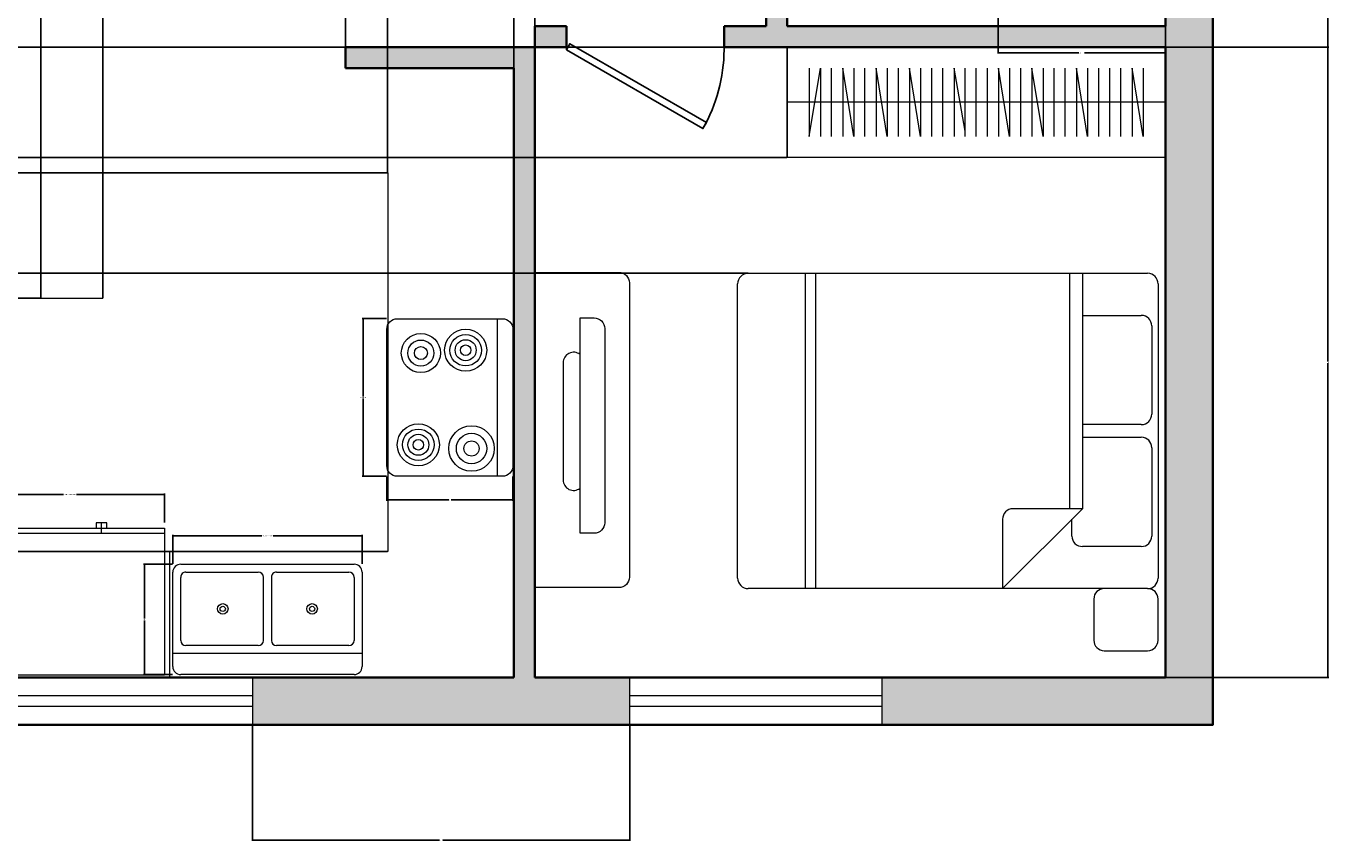
# Model space of a CAD drawing. Units: inches. Extents: x 2800 to 3283, y 1752 to 2114.
# Tile 5 of 6: x 3035 to 3283, y 1752 to 1907. Entities that reach past the tile are written whole.
import ezdxf

# ---------------------------------------------------------------- set-up
doc = ezdxf.new("R2010")
doc.units = ezdxf.units.IN
for name, color, linetype, lineweight in [('A-ANNO-DIMS', 2, 'Continuous', 18), ('A-DOOR', 3, 'Continuous', 25), ('A-EQPM', 8, 'Continuous', 18), ('A-FLOR-CASE', 8, 'Continuous', 18), ('A-FLOR-FIXT', 9, 'Continuous', 18), ('A-FURN', 9, 'Continuous', 18), ('A-GLAZ', 4, 'Continuous', 18), ('A-WALL', 7, 'Continuous', 35)]:
    doc.layers.add(name, color=color, linetype=linetype, lineweight=lineweight)
doc.layers.add('A-WALL-PATT', color=18, linetype='Continuous', lineweight=13, true_color=0x000000)
doc.styles.get("Standard").update_dxf_attribs({"font": 'arial.ttf'})
doc.dimstyles.get("Standard").update_dxf_attribs({"dimtxt": 0.18, "dimasz": 0.18, "dimexe": 0.18, "dimexo": 0.0625, "dimgap": 0.09, "dimtad": 0, "dimtih": 1, "dimtoh": 1, "dimdec": 4, "dimzin": 0, "dimdsep": 46, "dimtxsty": 'Standard', "dimcen": 0.09, "dimadec": 0, "dimazin": 0, "dimtfac": 1, "dimtdec": 4, "dimtofl": 0, "dimtmove": 0, "dimatfit": 3, "dimfxl": 1, "dimtolj": 1, "dimtzin": 0, "dimarcsym": 0})

# ---------------------------------------------------------------- blocks, each defined once
blk = doc.blocks.new('Range-Oven - 30 in top')
blk.add_line((0, -3), (30, -3))
blk.add_lwpolyline([(0, -22), (0, -2, -0.414214), (2, 0), (28, 0, -0.414214), (30, -2), (30, -22, -0.414214), (28, -24), (2, -24, -0.414214)], format="xyb", close=True)
for centre, radius in [((24.71, -7.88), 4.33), ((6, -9), 4), ((6, -9), 3), ((6, -9), 2), ((24.71, -7.88), 2.89), ((24.71, -7.88), 1.44), ((6, -9), 1), ((6.54, -17.52), 3.72), ((24, -18), 4), ((6.54, -17.52), 2.48), ((6.54, -17.52), 1.24), ((24, -18), 3), ((24, -18), 2), ((24, -18), 1)]:
    blk.add_circle(centre, radius)
blk = doc.blocks.new('Sink-double - 36 in top')
for p, q in [((-18, -4), (18, -4)), ((-0.75, -18.5), (-0.75, -6.5)), ((0.75, -6.5), (0.75, -18.5))]:
    blk.add_line(p, q)
for points in [[(-16.5, 0), (16.5, 0)], [(-18, -19.5), (-18, -1.5)], [(18, -1.5), (18, -19.5)], [(-16.5, -18.5), (-16.5, -6.5)], [(-15.5, -5.5), (-1.75, -5.5)], [(1.75, -5.5), (15.5, -5.5)], [(16.5, -6.5), (16.5, -18.5)], [(-1.75, -19.5), (-15.5, -19.5)], [(15.5, -19.5), (1.75, -19.5)], [(16.5, -21), (-16.5, -21)]]:
    blk.add_lwpolyline(points)
for centre, radius in [((-8.5, -12.5), 1), ((-8.5, -12.5), 0.5), ((8.5, -12.5), 1), ((8.5, -12.5), 0.5)]:
    blk.add_circle(centre, radius)
for centre, radius, start, end in [((-16.5, -1.5), 1.5, 90, 180), ((16.5, -1.5), 1.5, 0, 90), ((-15.5, -6.5), 1, 90, 180), ((-1.75, -6.5), 1, 0, 90), ((1.75, -6.5), 1, 90, 180), ((15.5, -6.5), 1, 0, 90), ((-16.5, -19.5), 1.5, 180, 270), ((-15.5, -18.5), 1, 180, 270), ((-1.75, -18.5), 1, 270, 0), ((1.75, -18.5), 1, 180, 270), ((15.5, -18.5), 1, 270, 0), ((16.5, -19.5), 1.5, 270, 0)]:
    blk.add_arc(centre, radius, start, end)
blk = doc.blocks.new('Bed - Queen')
for p, q in [((2, 0), (58, 0)), ((0, -78), (0, -2)), ((10, -1.2), (26.8, -1.2)), ((33.2, -1.2), (50, -1.2)), ((60, -2), (60, -78)), ((8, -14.4), (8, -3.2)), ((28.8, -3.2), (28.8, -14.4)), ((31.2, -14.4), (31.2, -3.2)), ((52, -3.2), (52, -14.4)), ((0, -14.4), (44.8, -14.4)), ((60, -29.6), (44.8, -14.4)), ((44.8, -14.4), (44.8, -27.6)), ((44.8, -16.8), (0, -16.8)), ((50, -16.4), (46.8, -16.4)), ((46.8, -29.6), (60, -29.6)), ((0, -65.18), (60, -65.18)), ((0, -67.18), (60, -67.18)), ((58, -80), (2, -80))]:
    blk.add_line(p, q)
for centre, start, end in [((58, -2), 0, 90), ((2, -2), 90, 180), ((10, -3.2), 90, 180), ((26.8, -3.2), 0, 90), ((33.2, -3.2), 90, 180), ((50, -3.2), 0, 90), ((50, -14.4), 270, 0), ((46.8, -27.6), 180, 270), ((2, -78), 180, 270), ((58, -78), 270, 0)]:
    blk.add_arc(centre, 2, start, end)
blk = doc.blocks.new('Refrigerator-2 door - 36 in top')
for p, q in [((0, -26.999999), (36, -26.999999)), ((12, -26.999999), (12, -28.999999)), ((11, -27.999999), (11, -28.999999)), ((11, -28.999999), (13, -28.999999)), ((13, -28.999999), (13, -27.999999))]:
    blk.add_line(p, q)
blk.add_lwpolyline([(0, -27.999999), (0, 0), (36, 0), (36, -27.999999)], close=True)
blk = doc.blocks.new('*U13')
for p, q in [((0, 0), (0, 6)), ((40, 0), (40, 6))]:
    blk.add_line(p, q)
blk.add_lwpolyline([(0, 0), (34.64, -20), (35.52, -18.48), (0.87, 1.52)], close=True)
blk.add_arc((0, 0), 40, 330, 0)
blk = doc.blocks.new('WARDROBE-72')
for p, q in [((10.5, 72), (10.5, 0)), ((17, 63.53), (4, 63.53)), ((17, 61.41), (4, 61.41)), ((17, 59.29), (4, 59.29)), ((17, 52.94), (4, 52.94)), ((17, 50.82), (4, 50.82)), ((17, 44.47), (4, 44.47)), ((17, 38.12), (4, 38.12)), ((17, 36), (4, 36)), ((17, 33.88), (4, 33.88)), ((17, 29.65), (4, 29.65)), ((17, 27.53), (4, 27.53)), ((17, 21.18), (4, 21.18)), ((17, 14.82), (4, 14.82)), ((17, 8.47), (4, 8.47))]:
    blk.add_line(p, q)
for points in [[(0, 0), (0, 72), (21, 72), (21, 0), (0, 0), (21, 0)], [(4, 67.76), (17, 67.76), (4, 65.65), (17, 65.65)], [(4, 57.18), (17, 57.18), (4, 55.06), (17, 55.06)], [(4, 48.71), (17, 48.71), (4, 46.59), (17, 46.59)], [(4, 42.35), (17, 42.35), (4, 40.23), (17, 40.23)], [(16.02, 33.88), (4, 31.76), (17, 31.76)], [(4, 25.41), (17, 25.41), (4, 23.29), (17, 23.29)], [(4, 19.06), (17, 19.06), (4, 16.94), (17, 16.94)], [(4, 12.71), (17, 12.71), (4, 10.59), (17, 10.59)], [(4, 4.23), (17, 4.23), (4, 6.35), (17, 6.35)]]:
    blk.add_lwpolyline(points)
blk = doc.blocks.new('WIN-48')
for p, q in [((0, 5.5), (48, 5.5)), ((0, 3.5), (48, 3.5))]:
    blk.add_line(p, q)
for points in [[(0, 0), (0, 9)], [(48, 9), (48, 0)]]:
    blk.add_lwpolyline(points)
blk = doc.blocks.new('MEDIA-CONSOLE-60')
for points in [[(0, 60), (16, 60, -0.414214), (18, 58), (18, 2, -0.414214), (16, 0), (0, 0)], [(8.61, 51.33), (11.3, 51.33, -0.414214), (13.3, 49.33), (13.3, 12.33, -0.414214), (11.3, 10.33), (8.61, 10.33)]]:
    blk.add_lwpolyline(points, format="xyb", close=True)
blk.add_lwpolyline([(8.61, 15.1), (8.61, 47.68)])
blk.add_lwpolyline([(8.61, 44.37, 0.62446), (5.38, 42.79), (5.38, 20.5, 0.62446), (8.61, 18.92, 0.62446)], format="xyb")
blk = doc.blocks.new('*D32')
at = {"layer": 'A-ANNO-DIMS', "color": 0, "lineweight": -2, "transparency": 16777216}
for p, q in [((3219.68, 1910.1), (3219.68, 1902.02)), ((3251.54, 1910.1), (3251.54, 1902.02)), ((3219.86, 1902.2), (3235.08, 1902.2)), ((3251.36, 1902.2), (3236.14, 1902.2))]:
    blk.add_line(p, q, dxfattribs=at)
at = {"layer": 'A-ANNO-DIMS', "color": 0, "transparency": 16777216}
for points in [[(3219.86, 1902.23), (3219.86, 1902.17), (3219.68, 1902.2)], [(3251.36, 1902.23), (3251.36, 1902.17), (3251.54, 1902.2)]]:
    blk.add_solid(points, dxfattribs=at)
at = {"layer": 'Defpoints', "color": 0, "transparency": 16777216}
for p in [(3219.68, 1910.16), (3251.54, 1910.16), (3251.54, 1902.2)]:
    blk.add_point(p, dxfattribs=at)
at = {"layer": 'A-ANNO-DIMS', "color": 0, "transparency": 16777216, "insert": (3235.61, 1902.2), "char_height": 0.18, "attachment_point": 5}
blk.add_mtext('\\A1;32 TYP.', dxfattribs=at)
blk = doc.blocks.new('*D37')
at = {"layer": 'A-ANNO-DIMS', "color": 0, "lineweight": -2, "transparency": 16777216}
for p, q in [((3103.32, 1851.58), (3098.7, 1851.58)), ((3098.88, 1851.4), (3098.88, 1836.76)), ((3098.88, 1821.76), (3098.88, 1836.39)), ((3103.32, 1821.58), (3098.7, 1821.58))]:
    blk.add_line(p, q, dxfattribs=at)
at = {"layer": 'A-ANNO-DIMS', "color": 0, "transparency": 16777216}
for points in [[(3098.85, 1851.4), (3098.91, 1851.4), (3098.88, 1851.58)], [(3098.85, 1821.76), (3098.91, 1821.76), (3098.88, 1821.58)]]:
    blk.add_solid(points, dxfattribs=at)
at = {"layer": 'Defpoints', "color": 0, "transparency": 16777216}
for p in [(3103.38, 1851.58), (3098.88, 1821.58), (3103.38, 1821.58)]:
    blk.add_point(p, dxfattribs=at)
at = {"layer": 'A-ANNO-DIMS', "color": 0, "transparency": 16777216, "insert": (3098.88, 1836.58), "char_height": 0.18, "attachment_point": 5}
blk.add_mtext('\\A1;RANGE 30', dxfattribs=at)
blk = doc.blocks.new('*D38')
at = {"layer": 'A-ANNO-DIMS', "color": 0, "lineweight": -2, "transparency": 16777216}
for p, q in [((3103.38, 1821.51), (3103.38, 1816.9)), ((3127.38, 1821.51), (3127.38, 1816.9)), ((3103.56, 1817.08), (3115.16, 1817.08)), ((3127.2, 1817.08), (3115.6, 1817.08))]:
    blk.add_line(p, q, dxfattribs=at)
at = {"layer": 'A-ANNO-DIMS', "color": 0, "transparency": 16777216}
for points in [[(3103.56, 1817.11), (3103.56, 1817.05), (3103.38, 1817.08)], [(3127.2, 1817.11), (3127.2, 1817.05), (3127.38, 1817.08)]]:
    blk.add_solid(points, dxfattribs=at)
at = {"layer": 'Defpoints', "color": 0, "transparency": 16777216}
for p in [(3103.38, 1821.58), (3127.38, 1821.58), (3127.38, 1817.08)]:
    blk.add_point(p, dxfattribs=at)
at = {"layer": 'A-ANNO-DIMS', "color": 0, "transparency": 16777216, "insert": (3115.38, 1817.08), "char_height": 0.18, "attachment_point": 5}
blk.add_mtext('\\A1;24', dxfattribs=at)
blk = doc.blocks.new('*D39')
at = {"layer": 'A-ANNO-DIMS', "color": 0, "lineweight": -2, "transparency": 16777216}
for p, q in [((3062.66, 1804.91), (3062.66, 1810.42)), ((3062.84, 1810.24), (3079.57, 1810.24)), ((3098.48, 1810.24), (3081.76, 1810.24)), ((3098.66, 1804.91), (3098.66, 1810.42))]:
    blk.add_line(p, q, dxfattribs=at)
at = {"layer": 'A-ANNO-DIMS', "color": 0, "transparency": 16777216}
for points in [[(3062.84, 1810.27), (3062.84, 1810.21), (3062.66, 1810.24)], [(3098.48, 1810.27), (3098.48, 1810.21), (3098.66, 1810.24)]]:
    blk.add_solid(points, dxfattribs=at)
at = {"layer": 'Defpoints', "color": 0, "transparency": 16777216}
for p in [(3062.66, 1810.24), (3062.66, 1804.84), (3098.66, 1804.84)]:
    blk.add_point(p, dxfattribs=at)
at = {"layer": 'A-ANNO-DIMS', "color": 0, "transparency": 16777216, "insert": (3080.66, 1810.24), "char_height": 0.18, "attachment_point": 5}
blk.add_mtext('\\A1;DOUBLE SINK 36', dxfattribs=at)
blk = doc.blocks.new('*D40')
at = {"layer": 'A-ANNO-DIMS', "color": 0, "lineweight": -2, "transparency": 16777216}
for p, q in [((3062.6, 1804.84), (3057.08, 1804.84)), ((3057.26, 1804.66), (3057.26, 1794.52)), ((3057.26, 1784.02), (3057.26, 1794.16)), ((3062.6, 1783.84), (3057.08, 1783.84))]:
    blk.add_line(p, q, dxfattribs=at)
at = {"layer": 'A-ANNO-DIMS', "color": 0, "transparency": 16777216}
for points in [[(3057.23, 1804.66), (3057.29, 1804.66), (3057.26, 1804.84)], [(3057.23, 1784.02), (3057.29, 1784.02), (3057.26, 1783.84)]]:
    blk.add_solid(points, dxfattribs=at)
at = {"layer": 'Defpoints', "color": 0, "transparency": 16777216}
for p in [(3062.66, 1804.84), (3057.26, 1783.84), (3062.66, 1783.84)]:
    blk.add_point(p, dxfattribs=at)
at = {"layer": 'A-ANNO-DIMS', "color": 0, "transparency": 16777216, "insert": (3057.26, 1794.34), "char_height": 0.18, "attachment_point": 5}
blk.add_mtext('\\A1;21', dxfattribs=at)
blk = doc.blocks.new('*D41')
at = {"layer": 'A-ANNO-DIMS', "color": 0, "lineweight": -2, "transparency": 16777216}
for p, q in [((3025.08, 1812.76), (3025.08, 1818.28)), ((3025.26, 1818.1), (3041.83, 1818.1)), ((3060.9, 1818.1), (3044.33, 1818.1)), ((3061.08, 1812.76), (3061.08, 1818.28))]:
    blk.add_line(p, q, dxfattribs=at)
at = {"layer": 'A-ANNO-DIMS', "color": 0, "transparency": 16777216}
for points in [[(3025.26, 1818.13), (3025.26, 1818.07), (3025.08, 1818.1)], [(3060.9, 1818.13), (3060.9, 1818.07), (3061.08, 1818.1)]]:
    blk.add_solid(points, dxfattribs=at)
at = {"layer": 'Defpoints', "color": 0, "transparency": 16777216}
for p in [(3025.08, 1818.1), (3025.08, 1812.7), (3061.08, 1812.7)]:
    blk.add_point(p, dxfattribs=at)
at = {"layer": 'A-ANNO-DIMS', "color": 0, "transparency": 16777216, "insert": (3043.08, 1818.1), "char_height": 0.18, "attachment_point": 5}
blk.add_mtext('\\A1;REFRIGERATOR 36', dxfattribs=at)
blk = doc.blocks.new('*D48')
at = {"layer": 'A-ANNO-DIMS', "color": 0, "lineweight": -2, "transparency": 16777216}
for p, q in [((3131.54, 1783.33), (3131.54, 2114.36)), ((3131.72, 2114.18), (3191.26, 2114.18)), ((3251.36, 2114.18), (3191.82, 2114.18)), ((3251.54, 1783.33), (3251.54, 2114.36))]:
    blk.add_line(p, q, dxfattribs=at)
at = {"layer": 'A-ANNO-DIMS', "color": 0, "transparency": 16777216}
for points in [[(3131.72, 2114.21), (3131.72, 2114.15), (3131.54, 2114.18)], [(3251.36, 2114.21), (3251.36, 2114.15), (3251.54, 2114.18)]]:
    blk.add_solid(points, dxfattribs=at)
at = {"layer": 'Defpoints', "color": 0, "transparency": 16777216}
for p in [(3251.54, 2114.18), (3131.54, 1783.27), (3251.54, 1783.27)]:
    blk.add_point(p, dxfattribs=at)
at = {"layer": 'A-ANNO-DIMS', "color": 0, "transparency": 16777216, "insert": (3191.54, 2114.18), "char_height": 0.18, "attachment_point": 5}
blk.add_mtext('\\A1;120', dxfattribs=at)
blk = doc.blocks.new('*D53')
at = {"layer": 'A-ANNO-DIMS', "color": 0, "lineweight": -2, "transparency": 16777216}
for p, q in [((3251.61, 1903.27), (3282.64, 1903.27)), ((3282.46, 1903.09), (3282.46, 1843.45)), ((3282.46, 1783.45), (3282.46, 1843.09)), ((3251.61, 1783.27), (3282.64, 1783.27))]:
    blk.add_line(p, q, dxfattribs=at)
at = {"layer": 'A-ANNO-DIMS', "color": 0, "transparency": 16777216}
for points in [[(3282.43, 1903.09), (3282.49, 1903.09), (3282.46, 1903.27)], [(3282.43, 1783.45), (3282.49, 1783.45), (3282.46, 1783.27)]]:
    blk.add_solid(points, dxfattribs=at)
at = {"layer": 'Defpoints', "color": 0, "transparency": 16777216}
for p in [(3251.54, 1903.27), (3282.46, 1903.27), (3251.54, 1783.27)]:
    blk.add_point(p, dxfattribs=at)
at = {"layer": 'A-ANNO-DIMS', "color": 0, "transparency": 16777216, "insert": (3282.46, 1843.27), "char_height": 0.18, "attachment_point": 5}
blk.add_mtext('\\A1;120', dxfattribs=at)
blk = doc.blocks.new('*D63')
at = {"layer": 'A-ANNO-DIMS', "color": 0, "lineweight": -2, "transparency": 16777216}
for p, q in [((3077.8, 1774.21), (3077.8, 1752.17)), ((3149.6, 1774.21), (3149.6, 1752.17)), ((3077.98, 1752.35), (3113.38, 1752.35)), ((3149.42, 1752.35), (3114.02, 1752.35))]:
    blk.add_line(p, q, dxfattribs=at)
at = {"layer": 'A-ANNO-DIMS', "color": 0, "transparency": 16777216}
for points in [[(3077.98, 1752.38), (3077.98, 1752.32), (3077.8, 1752.35)], [(3149.42, 1752.38), (3149.42, 1752.32), (3149.6, 1752.35)]]:
    blk.add_solid(points, dxfattribs=at)
at = {"layer": 'Defpoints', "color": 0, "transparency": 16777216}
for p in [(3077.8, 1774.27), (3149.6, 1774.27), (3149.6, 1752.35)]:
    blk.add_point(p, dxfattribs=at)
at = {"layer": 'A-ANNO-DIMS', "color": 0, "transparency": 16777216, "insert": (3113.7, 1752.35), "char_height": 0.18, "attachment_point": 5}
blk.add_mtext('\\A1;71.8', dxfattribs=at)
blk = doc.blocks.new('*D64')
at = {"layer": 'A-ANNO-DIMS', "color": 0, "lineweight": -2, "transparency": 16777216}
for p, q in [((2831.61, 1922.35), (3282.64, 1922.35)), ((3282.46, 1922.17), (3282.46, 1912.99)), ((3282.46, 1903.45), (3282.46, 1912.63)), ((2831.61, 1903.27), (3282.64, 1903.27))]:
    blk.add_line(p, q, dxfattribs=at)
at = {"layer": 'A-ANNO-DIMS', "color": 0, "transparency": 16777216}
for points in [[(3282.43, 1922.17), (3282.49, 1922.17), (3282.46, 1922.35)], [(3282.43, 1903.45), (3282.49, 1903.45), (3282.46, 1903.27)]]:
    blk.add_solid(points, dxfattribs=at)
at = {"layer": 'Defpoints', "color": 0, "transparency": 16777216}
for p in [(2831.54, 1922.35), (3282.46, 1922.35), (2831.54, 1903.27)]:
    blk.add_point(p, dxfattribs=at)
at = {"layer": 'A-ANNO-DIMS', "color": 0, "transparency": 16777216, "insert": (3282.46, 1912.81), "char_height": 0.18, "attachment_point": 5}
blk.add_mtext('\\A1;19.085', dxfattribs=at)
blk = doc.blocks.new('*D70')
at = {"layer": 'A-ANNO-DIMS', "color": 0, "lineweight": -2, "transparency": 16777216}
for p, q in [((3037.54, 1903.33), (3037.54, 2114.36)), ((3037.72, 2114.18), (3082.32, 2114.18)), ((3127.36, 2114.18), (3082.76, 2114.18)), ((3127.54, 1899.33), (3127.54, 2114.36))]:
    blk.add_line(p, q, dxfattribs=at)
at = {"layer": 'A-ANNO-DIMS', "color": 0, "transparency": 16777216}
for points in [[(3037.72, 2114.21), (3037.72, 2114.15), (3037.54, 2114.18)], [(3127.36, 2114.21), (3127.36, 2114.15), (3127.54, 2114.18)]]:
    blk.add_solid(points, dxfattribs=at)
at = {"layer": 'Defpoints', "color": 0, "transparency": 16777216}
for p in [(3127.54, 2114.18), (3037.54, 1903.27), (3127.54, 1899.27)]:
    blk.add_point(p, dxfattribs=at)
at = {"layer": 'A-ANNO-DIMS', "color": 0, "transparency": 16777216, "insert": (3082.54, 2114.18), "char_height": 0.18, "attachment_point": 5}
blk.add_mtext('\\A1;90', dxfattribs=at)
blk = doc.blocks.new('*D71')
at = {"layer": 'A-ANNO-DIMS', "color": 0, "lineweight": -2, "transparency": 16777216}
for p, q in [((3037.48, 1903.27), (2800.45, 1903.27)), ((2800.63, 1903.09), (2800.63, 1879.54)), ((2800.63, 1855.63), (2800.63, 1879.18)), ((3037.48, 1855.45), (2800.45, 1855.45))]:
    blk.add_line(p, q, dxfattribs=at)
at = {"layer": 'A-ANNO-DIMS', "color": 0, "transparency": 16777216}
for points in [[(2800.6, 1903.09), (2800.66, 1903.09), (2800.63, 1903.27)], [(2800.6, 1855.63), (2800.66, 1855.63), (2800.63, 1855.45)]]:
    blk.add_solid(points, dxfattribs=at)
at = {"layer": 'Defpoints', "color": 0, "transparency": 16777216}
for p in [(2800.63, 1903.27), (3037.54, 1903.27), (3037.54, 1855.45)]:
    blk.add_point(p, dxfattribs=at)
at = {"layer": 'A-ANNO-DIMS', "color": 0, "transparency": 16777216, "insert": (2800.63, 1879.36), "char_height": 0.18, "attachment_point": 5}
blk.add_mtext('\\A1;47.82', dxfattribs=at)
blk = doc.blocks.new('*D72')
at = {"layer": 'A-ANNO-DIMS', "color": 0, "lineweight": -2, "transparency": 16777216}
for p, q in [((3049.36, 1879.34), (3049.36, 2114.36)), ((3049.54, 2114.18), (3076.06, 2114.18)), ((3103.36, 2114.18), (3076.84, 2114.18)), ((3103.54, 1879.4), (3103.54, 2114.36))]:
    blk.add_line(p, q, dxfattribs=at)
at = {"layer": 'A-ANNO-DIMS', "color": 0, "transparency": 16777216}
for points in [[(3049.54, 2114.21), (3049.54, 2114.15), (3049.36, 2114.18)], [(3103.36, 2114.21), (3103.36, 2114.15), (3103.54, 2114.18)]]:
    blk.add_solid(points, dxfattribs=at)
at = {"layer": 'Defpoints', "color": 0, "transparency": 16777216}
for p in [(3103.54, 2114.18), (3049.36, 1879.28), (3103.54, 1879.34)]:
    blk.add_point(p, dxfattribs=at)
at = {"layer": 'A-ANNO-DIMS', "color": 0, "transparency": 16777216, "insert": (3076.45, 2114.18), "char_height": 0.18, "attachment_point": 5}
blk.add_mtext('\\A1;54.19', dxfattribs=at)
blk = doc.blocks.new('*D73')
at = {"layer": 'A-ANNO-DIMS', "color": 0, "lineweight": -2, "transparency": 16777216}
for p, q in [((3103.48, 1879.34), (2800.45, 1879.34)), ((2800.63, 1879.16), (2800.63, 1843.49)), ((2800.63, 1807.45), (2800.63, 1843.12)), ((3103.48, 1807.27), (2800.45, 1807.27))]:
    blk.add_line(p, q, dxfattribs=at)
at = {"layer": 'A-ANNO-DIMS', "color": 0, "transparency": 16777216}
for points in [[(2800.6, 1879.16), (2800.66, 1879.16), (2800.63, 1879.34)], [(2800.6, 1807.45), (2800.66, 1807.45), (2800.63, 1807.27)]]:
    blk.add_solid(points, dxfattribs=at)
at = {"layer": 'Defpoints', "color": 0, "transparency": 16777216}
for p in [(2800.63, 1879.34), (3103.54, 1879.34), (3103.54, 1807.27)]:
    blk.add_point(p, dxfattribs=at)
at = {"layer": 'A-ANNO-DIMS', "color": 0, "transparency": 16777216, "insert": (2800.63, 1843.31), "char_height": 0.18, "attachment_point": 5}
blk.add_mtext('\\A1;72.07', dxfattribs=at)
blk = doc.blocks.new('*D74')
at = {"layer": 'A-ANNO-DIMS', "color": 0, "lineweight": -2, "transparency": 16777216}
for p, q in [((3037.54, 1855.51), (3037.54, 2114.36)), ((3037.72, 2114.18), (3043, 2114.18)), ((3049.18, 2114.18), (3043.91, 2114.18)), ((3049.36, 1855.51), (3049.36, 2114.36))]:
    blk.add_line(p, q, dxfattribs=at)
at = {"layer": 'A-ANNO-DIMS', "color": 0, "transparency": 16777216}
for points in [[(3037.72, 2114.21), (3037.72, 2114.15), (3037.54, 2114.18)], [(3049.18, 2114.21), (3049.18, 2114.15), (3049.36, 2114.18)]]:
    blk.add_solid(points, dxfattribs=at)
at = {"layer": 'Defpoints', "color": 0, "transparency": 16777216}
for p in [(3049.36, 2114.18), (3037.54, 1855.45), (3049.36, 1855.45)]:
    blk.add_point(p, dxfattribs=at)
at = {"layer": 'A-ANNO-DIMS', "color": 0, "transparency": 16777216, "insert": (3043.45, 2114.18), "char_height": 0.18, "attachment_point": 5}
blk.add_mtext('\\A1;11.814', dxfattribs=at)
blk = doc.blocks.new('*D75')
at = {"layer": 'A-ANNO-DIMS', "color": 0, "lineweight": -2, "transparency": 16777216}
for p, q in [((3095.54, 1899.33), (3095.54, 2114.36)), ((3095.72, 2114.18), (3111.33, 2114.18)), ((3127.36, 2114.18), (3111.76, 2114.18)), ((3127.54, 1899.33), (3127.54, 2114.36))]:
    blk.add_line(p, q, dxfattribs=at)
at = {"layer": 'A-ANNO-DIMS', "color": 0, "transparency": 16777216}
for points in [[(3095.72, 2114.21), (3095.72, 2114.15), (3095.54, 2114.18)], [(3127.36, 2114.21), (3127.36, 2114.15), (3127.54, 2114.18)]]:
    blk.add_solid(points, dxfattribs=at)
at = {"layer": 'Defpoints', "color": 0, "transparency": 16777216}
for p in [(3127.54, 2114.18), (3095.54, 1899.27), (3127.54, 1899.27)]:
    blk.add_point(p, dxfattribs=at)
at = {"layer": 'A-ANNO-DIMS', "color": 0, "transparency": 16777216, "insert": (3111.54, 2114.18), "char_height": 0.18, "attachment_point": 5}
blk.add_mtext('\\A1;32', dxfattribs=at)
blk = doc.blocks.new('*D76')
at = {"layer": 'A-ANNO-DIMS', "color": 0, "lineweight": -2, "transparency": 16777216}
for p, q in [((3095.48, 1903.27), (2800.45, 1903.27)), ((2800.63, 1903.09), (2800.63, 1891.49)), ((2800.63, 1879.52), (2800.63, 1891.12)), ((3103.48, 1879.34), (2800.45, 1879.34))]:
    blk.add_line(p, q, dxfattribs=at)
at = {"layer": 'A-ANNO-DIMS', "color": 0, "transparency": 16777216}
for points in [[(2800.6, 1903.09), (2800.66, 1903.09), (2800.63, 1903.27)], [(2800.6, 1879.52), (2800.66, 1879.52), (2800.63, 1879.34)]]:
    blk.add_solid(points, dxfattribs=at)
at = {"layer": 'Defpoints', "color": 0, "transparency": 16777216}
for p in [(3095.54, 1903.27), (2800.63, 1879.34), (3103.54, 1879.34)]:
    blk.add_point(p, dxfattribs=at)
at = {"layer": 'A-ANNO-DIMS', "color": 0, "transparency": 16777216, "insert": (2800.63, 1891.31), "char_height": 0.18, "attachment_point": 5}
blk.add_mtext('\\A1;23.93', dxfattribs=at)
blk = doc.blocks.new('*D84')
at = {"layer": 'A-ANNO-DIMS', "color": 0, "lineweight": -2, "transparency": 16777216}
for p, q in [((3179.48, 1882.27), (2800.45, 1882.27)), ((2800.63, 1882.09), (2800.63, 1871.42)), ((2800.63, 1860.39), (2800.63, 1871.06)), ((3172.07, 1860.21), (2800.45, 1860.21))]:
    blk.add_line(p, q, dxfattribs=at)
at = {"layer": 'A-ANNO-DIMS', "color": 0, "transparency": 16777216}
for points in [[(2800.6, 1882.09), (2800.66, 1882.09), (2800.63, 1882.27)], [(2800.6, 1860.39), (2800.66, 1860.39), (2800.63, 1860.21)]]:
    blk.add_solid(points, dxfattribs=at)
at = {"layer": 'Defpoints', "color": 0, "transparency": 16777216}
for p in [(3179.54, 1882.27), (2800.63, 1860.21), (3172.14, 1860.21)]:
    blk.add_point(p, dxfattribs=at)
at = {"layer": 'A-ANNO-DIMS', "color": 0, "transparency": 16777216, "insert": (2800.63, 1871.24), "char_height": 0.18, "attachment_point": 5}
blk.add_mtext('\\A1;22.06', dxfattribs=at)

msp = doc.modelspace()

# ---------------------------------------------------------------- hatches: boundary and pattern name
at = {"layer": 'A-WALL-PATT'}
h = msp.add_hatch(color=256, dxfattribs=at)
h.dxf.hatch_style = 1
h.paths.add_polyline_path([(3260.5432, 1926.3971), (3251.5432, 1926.3971), (3251.5432, 1910.1641), (3251.5432, 1907.2695), (3179.5432, 1907.2695), (3179.5432, 1933.2695), (3175.5432, 1933.2695), (3175.5432, 1907.2695), (3167.5432, 1907.2695), (3167.5432, 1903.2695), (3251.5432, 1903.2695), (3251.5432, 1882.2695), (3251.5432, 1783.2695), (3197.6001, 1783.2695), (3197.6001, 1774.2695), (3260.5432, 1774.2695)])
h = msp.add_hatch(color=256, dxfattribs=at)
h.dxf.hatch_style = 1
h.paths.add_polyline_path([(3137.5432, 1907.2695), (3131.5432, 1907.2695), (3131.5432, 1903.2695), (3137.5432, 1903.2695)])
h = msp.add_hatch(color=256, dxfattribs=at)
h.dxf.hatch_style = 1
h.paths.add_polyline_path([(3149.6001, 1783.2695), (3131.5432, 1783.2695), (3131.5432, 1903.2695), (3095.5432, 1903.2695), (3095.5432, 1899.2695), (3127.5432, 1899.2695), (3127.5432, 1783.2695), (3077.8011, 1783.2695), (3077.8011, 1774.2695), (3149.6001, 1774.2695)])

# ---------------------------------------------------------------- linework, layer by layer
at = {"layer": 'A-FLOR-CASE'}
for p, q in [((3037.5432, 1903.2695), (3037.5432, 1855.4517)), ((3095.5432, 1903.2695), (3037.5432, 1903.2695)), ((3103.5432, 1903.3668), (3103.5432, 1903.3409)), ((3049.3576, 1879.2823), (3103.5432, 1879.3408)), ((3049.3576, 1855.4517), (3049.3576, 1879.2823)), ((3103.5432, 1879.3408), (3103.5432, 1807.2695)), ((3127.5432, 1879.3668), (3127.5691, 1879.3668)), ((3037.5432, 1855.4517), (3049.3576, 1855.4517)), ((3103.5432, 1807.2695), (3061.9998, 1807.2695)), ((3061.9998, 1807.2695), (3061.9998, 1783.2695))]:
    msp.add_line(p, q, dxfattribs=at)
at = {"layer": 'A-FURN'}
msp.add_lwpolyline([(3248.1372, 1800.2087), (3239.9044, 1800.2087, 0.41421356), (3237.9044, 1798.2087), (3237.9044, 1790.3752, 0.41421356), (3239.9044, 1788.3752), (3248.1372, 1788.3752, 0.41421356), (3250.1372, 1790.3752), (3250.1372, 1798.2087, 0.41421356)], format="xyb", close=True, dxfattribs=at)
at = {"layer": 'A-WALL'}
for p, q in [((3251.5432, 1963.2695), (3251.5432, 1907.2695)), ((3175.5432, 1933.2695), (3175.5432, 1907.2695)), ((3179.5432, 1933.2695), (3179.5432, 1907.2695)), ((3131.5432, 1903.2695), (3131.5432, 1907.2695)), ((3131.5432, 1907.2695), (3137.5432, 1907.2695)), ((3137.5432, 1907.2695), (3137.5432, 1903.2695)), ((3175.5432, 1907.2695), (3167.5432, 1907.2695)), ((3167.5432, 1903.2695), (3167.5432, 1907.2695)), ((3251.5432, 1907.2695), (3179.5432, 1907.2695)), ((3125.5432, 1903.2695), (3095.5432, 1903.2695)), ((3095.5432, 1903.2695), (3095.5432, 1899.2695)), ((3125.5432, 1903.2695), (3131.5432, 1903.2695)), ((3131.5432, 1903.2695), (3131.5432, 1783.2695)), ((3131.5432, 1903.2695), (3137.5432, 1903.2695)), ((3251.5432, 1903.2695), (3167.5432, 1903.2695)), ((3251.5432, 1903.2695), (3251.5432, 1783.2695)), ((3095.5432, 1899.2695), (3127.5432, 1899.2695)), ((3127.5432, 1899.2695), (3127.5432, 1783.2695)), ((3127.5432, 1783.2695), (3015.5432, 1783.2695)), ((3251.5432, 1783.2695), (3131.5432, 1783.2695))]:
    msp.add_line(p, q, dxfattribs=at)
msp.add_lwpolyline([(2967.5432, 1774.2695), (2822.5432, 1774.2695), (2822.5432, 2092.2695), (3260.5432, 2092.2695), (3260.5432, 1774.2695), (3015.5432, 1774.2695)], dxfattribs=at)

# ---------------------------------------------------------------- block references
at = {"layer": 'A-DOOR', "xscale": 0.75, "yscale": 0.75, "zscale": 0.75}
msp.add_blockref('*U13', (3137.5432, 1902.7695), dxfattribs=at)
at = {"layer": 'A-EQPM'}
for name, p, rotation in [('Range-Oven - 30 in top', (3127.3819, 1851.576), 270), ('Refrigerator-2 door - 36 in top', (3061.0792, 1783.7005), 180)]:
    msp.add_blockref(name, p, dxfattribs=dict(at, rotation=rotation))
at = {"layer": 'A-FLOR-CASE', "rotation": 270}
msp.add_blockref('WARDROBE-72', (3179.5437, 1903.2697), dxfattribs=at)
at = {"layer": 'A-FLOR-FIXT', "rotation": 180}
msp.add_blockref('Sink-double - 36 in top', (3080.6637, 1783.8438), dxfattribs=at)
at = {"layer": 'A-FURN'}
msp.add_blockref('MEDIA-CONSOLE-60', (3131.543, 1800.3915), dxfattribs=at)
at = {"layer": 'A-FURN', "rotation": 270}
msp.add_blockref('Bed - Queen', (3250.1372, 1860.2087), dxfattribs=at)
at = {"layer": 'A-GLAZ', "rotation": 180}
for p in [(3077.801, 1783.269), (3197.6, 1783.269)]:
    msp.add_blockref('WIN-48', p, dxfattribs=at)

# ---------------------------------------------------------------- dimensions: what is measured, and where the dimension line sits
at = {"layer": 'A-ANNO-DIMS'}
for base, p1, p2, override, picture, middle in [((3127.5432, 2114.1845), (3037.5432, 1903.2695), (3127.5432, 1899.2695), {"dimdec": 0, "dimlfac": 1, "dimrnd": 0, "dimzin": 0, "dimdsep": 46, "dimlunit": 2}, '*D70', (3082.5432, 2114.1845)), ((3049.3576, 2114.1845), (3037.5432, 1855.4517), (3049.3576, 1855.4517), {"dimdec": 3, "dimlfac": 1, "dimrnd": 0, "dimzin": 0, "dimdsep": 46, "dimlunit": 2}, '*D74', (3043.4504, 2114.1845)), ((3103.5432, 2114.1845), (3049.3576, 1879.2823), (3103.5432, 1879.3408), {"dimdec": 2, "dimlfac": 1, "dimrnd": 0, "dimzin": 0, "dimdsep": 46, "dimlunit": 2}, '*D72', (3076.4504, 2114.1845)), ((3127.5432, 2114.1845), (3095.5432, 1899.2695), (3127.5432, 1899.2695), {"dimdec": 0, "dimlfac": 1, "dimrnd": 0, "dimzin": 0, "dimdsep": 46, "dimlunit": 2}, '*D75', (3111.5432, 2114.1845)), ((3251.5432, 2114.1845), (3131.5432, 1783.2695), (3251.5432, 1783.2695), {"dimdec": 0, "dimlfac": 1, "dimrnd": 0, "dimzin": 0, "dimdsep": 46, "dimlunit": 2}, '*D48', (3191.5432, 2114.1845)), ((3127.3819, 1817.076), (3103.3819, 1821.576), (3127.3819, 1821.576), {"dimdec": 0, "dimlfac": 1, "dimrnd": 0, "dimzin": 0, "dimdsep": 46, "dimlunit": 2}, '*D38', (3115.3819, 1817.076)), ((3149.6001, 1752.3545), (3077.8011, 1774.2695), (3149.6001, 1774.2695), {"dimdec": 1, "dimlfac": 1, "dimrnd": 0, "dimzin": 0, "dimdsep": 46, "dimlunit": 2}, '*D63', (3113.7006, 1752.3545))]:
    dim = msp.add_linear_dim(base=base, p1=p1, p2=p2, dimstyle='Standard', override=override, dxfattribs=at)
    dim.commit()
    dim.dimension.update_dxf_attribs({"geometry": picture, "text_midpoint": middle})
for base, p1, p2, angle, override, picture, middle in [((3282.4582, 1922.3547), (2831.5432, 1903.2695), (2831.5432, 1922.3547), 90, {"dimdec": 3, "dimlfac": 1, "dimrnd": 0, "dimzin": 0, "dimdsep": 46, "dimlunit": 2}, '*D64', (3282.4582, 1912.8121)), ((2800.6282, 1903.2695), (3037.5432, 1855.4517), (3037.5432, 1903.2695), 90, {"dimdec": 2, "dimlfac": 1, "dimrnd": 0, "dimzin": 0, "dimdsep": 46, "dimlunit": 2}, '*D71', (2800.6282, 1879.3606)), ((2800.6282, 1879.3408), (3095.5432, 1903.2695), (3103.5432, 1879.3408), 90, {"dimdec": 2, "dimlfac": 1, "dimrnd": 0, "dimzin": 0, "dimdsep": 46, "dimlunit": 2}, '*D76', (2800.6282, 1891.3052)), ((3282.4582, 1903.2695), (3251.5432, 1783.2695), (3251.5432, 1903.2695), 90, {"dimdec": 0, "dimlfac": 1, "dimrnd": 0, "dimzin": 0, "dimdsep": 46, "dimlunit": 2}, '*D53', (3282.4582, 1843.2695)), ((2800.6282, 1860.2087), (3179.5432, 1882.2695), (3172.1372, 1860.2087), 90, {"dimdec": 2, "dimlfac": 1, "dimrnd": 0, "dimzin": 0, "dimdsep": 46, "dimlunit": 2}, '*D84', (2800.6282, 1871.2391)), ((2800.6282, 1879.3408), (3103.5432, 1807.2695), (3103.5432, 1879.3408), 90, {"dimdec": 2, "dimlfac": 1, "dimrnd": 0, "dimzin": 0, "dimdsep": 46, "dimlunit": 2}, '*D73', (2800.6282, 1843.3052)), ((3057.2637, 1783.8438), (3062.6637, 1804.8438), (3062.6637, 1783.8438), 270, {"dimdec": 0, "dimlfac": 1, "dimrnd": 0, "dimzin": 0, "dimdsep": 46, "dimlunit": 2}, '*D40', (3057.2637, 1794.3438))]:
    dim = msp.add_linear_dim(base=base, p1=p1, p2=p2, angle=angle, dimstyle='Standard', override=override, dxfattribs=at)
    dim.commit()
    dim.dimension.update_dxf_attribs({"geometry": picture, "text_midpoint": middle})
dim = msp.add_linear_dim(base=(3251.5432, 1902.1983), p1=(3219.68, 1910.1641), p2=(3251.5432, 1910.1641), text='<> TYP.', dimstyle='Standard', override={"dimdec": 0, "dimlfac": 1, "dimrnd": 0, "dimzin": 0, "dimdsep": 46, "dimlunit": 2}, dxfattribs=at)
dim.commit()
dim.dimension.update_dxf_attribs({"geometry": '*D32', "text_midpoint": (3235.6116, 1902.1983)})
for base, p1, p2, angle, text, picture, middle in [((3098.8819, 1821.576), (3103.3819, 1851.576), (3103.3819, 1821.576), 270, 'RANGE <>', '*D37', (3098.8819, 1836.576)), ((3025.0792, 1818.1005), (3061.0792, 1812.7005), (3025.0792, 1812.7005), 180, 'REFRIGERATOR <>', '*D41', (3043.0792, 1818.1005)), ((3062.6637, 1810.2438), (3098.6637, 1804.8438), (3062.6637, 1804.8438), 180, 'DOUBLE SINK <>', '*D39', (3080.6637, 1810.2438))]:
    dim = msp.add_linear_dim(base=base, p1=p1, p2=p2, angle=angle, text=text, dimstyle='Standard', override={"dimdec": 0, "dimlfac": 1, "dimrnd": 0, "dimzin": 0, "dimdsep": 46, "dimlunit": 2}, dxfattribs=at)
    dim.commit()
    dim.dimension.update_dxf_attribs({"geometry": picture, "text_midpoint": middle})

doc.saveas('drawing.dxf')
